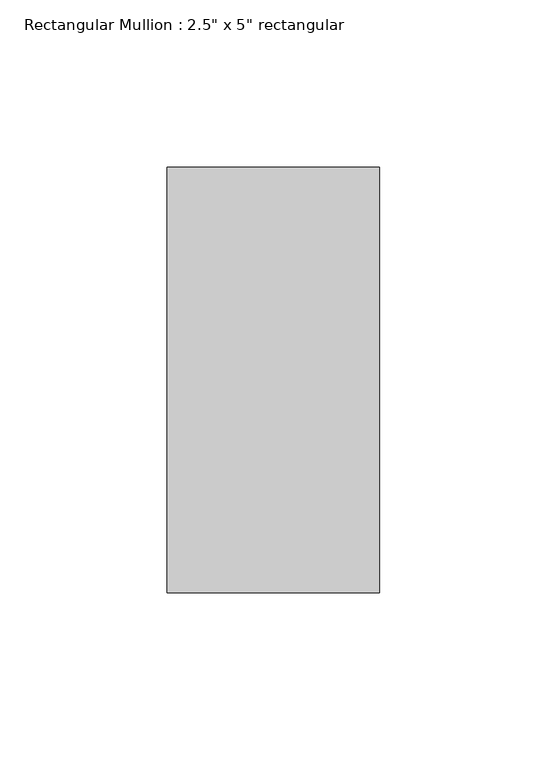
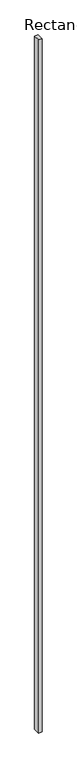
"""IFC4 building model written with IfcOpenShell, lengths in millimetres: member geometry."""

from ifc_helpers import new_model, si_unit, frame, origin, place, context, project, spatial, polyline, outline, extrude, source, transform, mapped, element, save


def member_315671ef(model_context):
    return source(origin(), model_context, "Body", "SweptSolid", [
        extrude(outline(polyline([(0.0, 63.5), (0.0, -63.5), (-63.5, -63.5), (-63.5, 63.5), (0.0, 63.5)])), frame((0.0, 0.0, -13741.4), z_axis=(0.0, 0.0, 1.0), x_axis=(1.0, 0.0, 0.0)), (0.0, 0.0, 1.0), 13741.4),
    ])


if __name__ == "__main__":
    model = new_model("IFC4")
    model_context = context("Model", 3, world=origin())
    ifc_project = project(units=[si_unit("LENGTHUNIT", "METRE", prefix="MILLI")], contexts=[model_context])
    site = spatial("IfcSite", under=ifc_project)
    building = spatial("IfcBuilding", under=site)
    placement = place(None, origin())
    member_shape = member_315671ef(model_context)
    element("IfcMember", 1, ObjectType="Rectangular Mullion : 2.5\" x 5\" rectangular", at=placement, inside=building, context=model_context, shape_type="MappedRepresentation", body=[
        mapped(member_shape, transform((0.0, 0.0, 0.0), x_axis=(1.0, 0.0, 0.0), y_axis=(0.0, 1.0, 0.0), z_axis=(0.0, 0.0, 1.0))),
    ])
    save(model, "model.ifc")

# Revit data of these elements
# Type "Rectangular Mullion : 2.5\" x 5\" rectangular"
#   built-in parameter 1007304 = 0.416667 (stored number, unit not read)
#   built-in parameter 1007301 = 0.104167 (stored number, unit not read)
#   built-in parameter 1007300 = 0.104167 (stored number, unit not read)
# Element 1 (IfcMember, "Rectangular Mullion : 2.5\" x 5\" rectangular")
#   Materials on its faces: "Aluminum"
# Materials
#   "Aluminum": class "Metal", colour RGB 247 247 247, transparency 0, Description = "Aluminum 6061", Cost = 0
